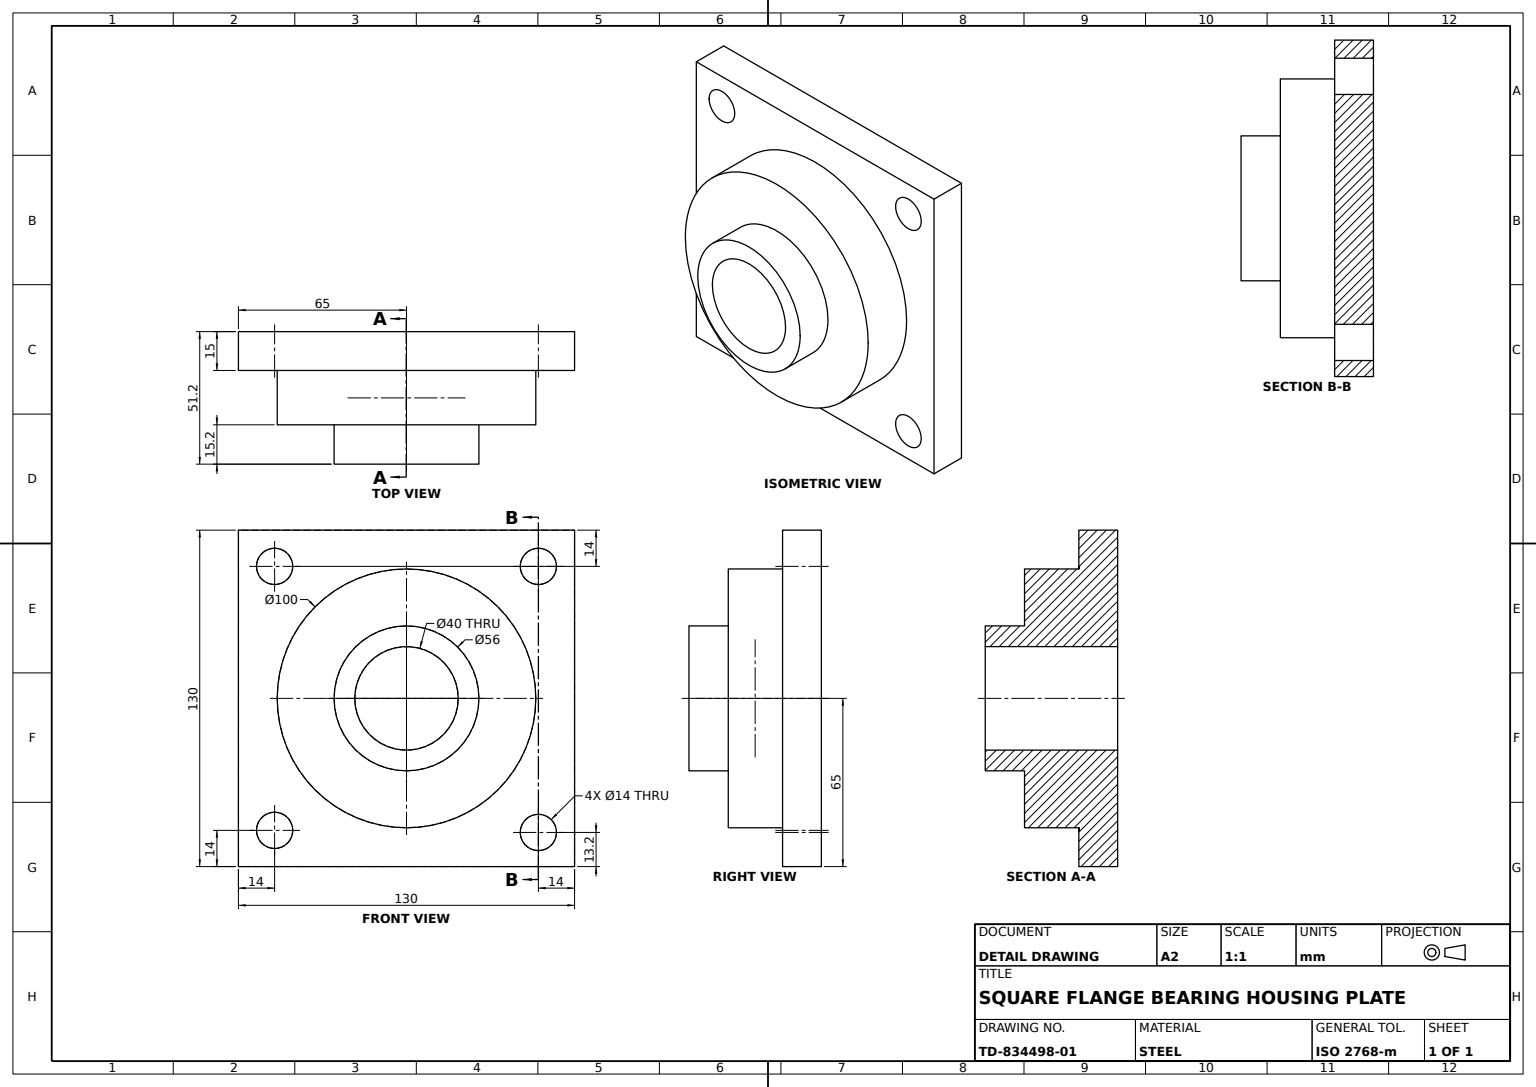
from build123d import *

# Parameters (mm, degrees)
FLANGE_PLATE_SKETCH_W         = 130
FLANGE_PLATE_SKETCH_H         = 130
FLANGE_PLATE_130X130X15_DEPTH = 15
HUB_SKETCH_100_R              = 50
HUB_100_DEPTH                 = 21
SPIGOT_SKETCH_56_R            = 28
SPIGOT_56_DEPTH               = 15.2
BORE_SKETCH_40_R              = 20
BORE_40_DEPTH                 = 51.2
MOUNTING_HOLES_SKETCH_R       = 7
MOUNTING_HOLES_4X_14_DEPTH    = 15


with BuildPart() as part:
    # Flange Plate Sketch → Flange Plate 130x130x15 (new body)
    with BuildSketch(Plane.XY):
        with Locations((65, 65)):
            Rectangle(FLANGE_PLATE_SKETCH_W, FLANGE_PLATE_SKETCH_H)
    extrude(amount=FLANGE_PLATE_130X130X15_DEPTH)

    # Hub Sketch Ø100 → Hub Ø100 (add)
    with BuildSketch(Plane.XY.offset(15)):
        with Locations(Location((65, 65, 0), (0, 0, 180))):
            Circle(HUB_SKETCH_100_R)
    extrude(amount=HUB_100_DEPTH)

    # Spigot Sketch Ø56 → Spigot Ø56 (add)
    with BuildSketch(Plane.XY.offset(36)):
        with Locations(Location((65, 65, 0), (0, 0, 180))):
            Circle(SPIGOT_SKETCH_56_R)
    extrude(amount=SPIGOT_56_DEPTH)

    # Bore Sketch Ø40 → Bore Ø40 (cut)
    with BuildSketch(Plane.XY.offset(51.2)):
        with Locations((65, 65)):
            Circle(BORE_SKETCH_40_R)
    extrude(amount=-BORE_40_DEPTH, mode=Mode.SUBTRACT)

    # Mounting Holes Sketch → Mounting Holes 4xØ14 (cut)
    with BuildSketch(Plane.XY.offset(15)):
        with Locations((116, 116)):
            Circle(MOUNTING_HOLES_SKETCH_R)
        with Locations((14, 116)):
            Circle(MOUNTING_HOLES_SKETCH_R)
        with Locations((14, 14)):
            Circle(MOUNTING_HOLES_SKETCH_R)
        with Locations((116, 13.196511798)):
            Circle(MOUNTING_HOLES_SKETCH_R)
    extrude(amount=-MOUNTING_HOLES_4X_14_DEPTH, mode=Mode.SUBTRACT)


solid = part.part
